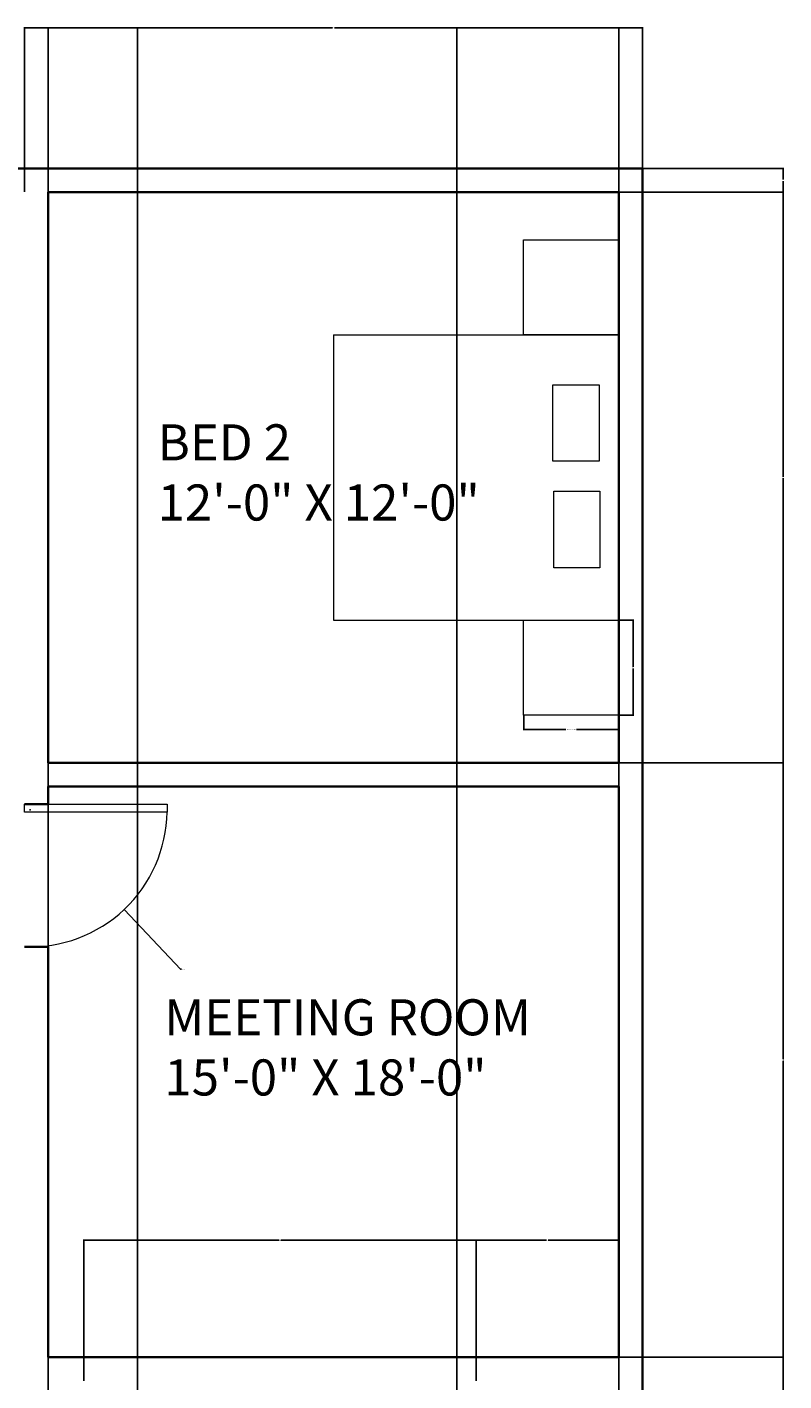
# Model space of a CAD drawing. Units: inches. Extents: x 4468 to 4972, y 2758 to 3538.
# Tile 4 of 4: x 4781 to 4972, y 3196 to 3538. Entities that reach past the tile are written whole.
import ezdxf

# ---------------------------------------------------------------- set-up
doc = ezdxf.new("R2010")
doc.units = ezdxf.units.IN
for name, color, linetype, lineweight in [('A-ANNO-DIMS', 2, 'Continuous', 18), ('A-AREA-IDEN', 7, 'Continuous', 18), ('A-DOOR', 4, 'Continuous', 18), ('A-FURN', 8, 'Continuous', 15), ('A-WALL', 7, 'Continuous', 35)]:
    doc.layers.add(name, color=color, linetype=linetype, lineweight=lineweight)
doc.styles.get("Standard").update_dxf_attribs({"font": 'arial.ttf'})
doc.dimstyles.get("Standard").update_dxf_attribs({"dimtxt": 0.18, "dimasz": 0.18, "dimexe": 0.18, "dimexo": 0.0625, "dimgap": 0.09, "dimtad": 0, "dimtih": 1, "dimtoh": 1, "dimdec": 4, "dimzin": 0, "dimdsep": 46, "dimtxsty": 'Standard', "dimcen": 0.09, "dimadec": 0, "dimazin": 0, "dimtfac": 1, "dimtdec": 4, "dimtofl": 0, "dimtmove": 0, "dimatfit": 3, "dimfxl": 1, "dimtolj": 1, "dimtzin": 0, "dimarcsym": 0})

# ---------------------------------------------------------------- blocks, each defined once
blk = doc.blocks.new('DOOR-LEAF-36IN')
for p, q in [((0, 0), (0, 36)), ((0, 36), (2, 36)), ((2, 36), (2, 0)), ((2, 0), (0, 0))]:
    blk.add_line(p, q)
blk = doc.blocks.new('BED-FRAME-72X72')
for p, q in [((0, 72), (0, 0)), ((0, 72), (72, 72)), ((0, 0), (72, 0))]:
    blk.add_line(p, q)
blk = doc.blocks.new('BED-PILLOW-PAIR')
for points in [[(0, 46.15), (11.65, 46.15), (11.65, 26.85), (0, 26.85)], [(0.18, 19.3), (11.83, 19.3), (11.83, 0), (0.18, 0)]]:
    blk.add_lwpolyline(points, close=True)
blk = doc.blocks.new('NIGHTSTAND-24X24')
blk.add_lwpolyline([(24, 24), (24, 0), (0, 0), (0, 24)], close=True)
blk = doc.blocks.new('*D19')
at = {"layer": 'A-ANNO-DIMS', "color": 0, "lineweight": -2, "transparency": 16777216}
for p, q in [((4906.18, 3364.1), (4906.18, 3360.38)), ((4930.18, 3364.1), (4930.18, 3360.38)), ((4906.36, 3360.56), (4916.8, 3360.56)), ((4930, 3360.56), (4919.55, 3360.56))]:
    blk.add_line(p, q, dxfattribs=at)
at = {"layer": 'A-ANNO-DIMS', "color": 0, "transparency": 16777216}
for points in [[(4906.36, 3360.59), (4906.36, 3360.53), (4906.18, 3360.56)], [(4930, 3360.59), (4930, 3360.53), (4930.18, 3360.56)]]:
    blk.add_solid(points, dxfattribs=at)
at = {"layer": 'Defpoints', "color": 0, "transparency": 16777216}
for p in [(4906.18, 3364.16), (4930.18, 3364.16), (4930.18, 3360.56)]:
    blk.add_point(p, dxfattribs=at)
at = {"layer": 'A-ANNO-DIMS', "color": 0, "transparency": 16777216, "insert": (4918.18, 3360.56), "char_height": 0.18, "attachment_point": 5}
blk.add_mtext('\\A1;NIGHTSTAND 24 TYP.', dxfattribs=at)
blk = doc.blocks.new('*D20')
at = {"layer": 'A-ANNO-DIMS', "color": 0, "lineweight": -2, "transparency": 16777216}
for p, q in [((4930.24, 3388.16), (4933.96, 3388.16)), ((4933.78, 3387.98), (4933.78, 3376.34)), ((4933.78, 3364.34), (4933.78, 3375.98)), ((4930.24, 3364.16), (4933.96, 3364.16))]:
    blk.add_line(p, q, dxfattribs=at)
at = {"layer": 'A-ANNO-DIMS', "color": 0, "transparency": 16777216}
for points in [[(4933.75, 3387.98), (4933.81, 3387.98), (4933.78, 3388.16)], [(4933.75, 3364.34), (4933.81, 3364.34), (4933.78, 3364.16)]]:
    blk.add_solid(points, dxfattribs=at)
at = {"layer": 'Defpoints', "color": 0, "transparency": 16777216}
for p in [(4930.18, 3388.16), (4933.78, 3388.16), (4930.18, 3364.16)]:
    blk.add_point(p, dxfattribs=at)
at = {"layer": 'A-ANNO-DIMS', "color": 0, "transparency": 16777216, "insert": (4933.78, 3376.16), "char_height": 0.18, "attachment_point": 5}
blk.add_mtext('\\A1;24 TYP.', dxfattribs=at)
blk = doc.blocks.new('*D40')
at = {"layer": 'A-ANNO-DIMS', "color": 0, "lineweight": -2, "transparency": 16777216}
for p, q in [((4780.18, 3496.22), (4780.18, 3537.84)), ((4780.36, 3537.66), (4857.9, 3537.66)), ((4936, 3537.66), (4858.46, 3537.66)), ((4936.18, 3502.22), (4936.18, 3537.84))]:
    blk.add_line(p, q, dxfattribs=at)
at = {"layer": 'A-ANNO-DIMS', "color": 0, "transparency": 16777216}
for points in [[(4780.36, 3537.69), (4780.36, 3537.63), (4780.18, 3537.66)], [(4936, 3537.69), (4936, 3537.63), (4936.18, 3537.66)]]:
    blk.add_solid(points, dxfattribs=at)
at = {"layer": 'Defpoints', "color": 0, "transparency": 16777216}
for p in [(4936.18, 3537.66), (4936.18, 3502.16), (4780.18, 3496.16)]:
    blk.add_point(p, dxfattribs=at)
at = {"layer": 'A-ANNO-DIMS', "color": 0, "transparency": 16777216, "insert": (4858.18, 3537.66), "char_height": 0.18, "attachment_point": 5}
blk.add_mtext('\\A1;156', dxfattribs=at)
blk = doc.blocks.new('*D43')
at = {"layer": 'A-ANNO-DIMS', "color": 0, "lineweight": -2, "transparency": 16777216}
for p, q in [((4930.24, 3496.16), (4971.86, 3496.16)), ((4971.68, 3495.98), (4971.68, 3424.34)), ((4971.68, 3352.34), (4971.68, 3423.98)), ((4930.24, 3352.16), (4971.86, 3352.16))]:
    blk.add_line(p, q, dxfattribs=at)
at = {"layer": 'A-ANNO-DIMS', "color": 0, "transparency": 16777216}
for points in [[(4971.65, 3495.98), (4971.71, 3495.98), (4971.68, 3496.16)], [(4971.65, 3352.34), (4971.71, 3352.34), (4971.68, 3352.16)]]:
    blk.add_solid(points, dxfattribs=at)
at = {"layer": 'Defpoints', "color": 0, "transparency": 16777216}
for p in [(4930.18, 3496.16), (4971.68, 3496.16), (4930.18, 3352.16)]:
    blk.add_point(p, dxfattribs=at)
at = {"layer": 'A-ANNO-DIMS', "color": 0, "transparency": 16777216, "insert": (4971.68, 3424.16), "char_height": 0.18, "attachment_point": 5}
blk.add_mtext('\\A1;144', dxfattribs=at)
blk = doc.blocks.new('*D44')
at = {"layer": 'A-ANNO-DIMS', "color": 0, "lineweight": -2, "transparency": 16777216}
for p, q in [((4930.24, 3352.16), (4971.86, 3352.16)), ((4971.68, 3351.98), (4971.68, 3277.34)), ((4971.68, 3202.34), (4971.68, 3276.98)), ((4930.24, 3202.16), (4971.86, 3202.16))]:
    blk.add_line(p, q, dxfattribs=at)
at = {"layer": 'A-ANNO-DIMS', "color": 0, "transparency": 16777216}
for points in [[(4971.65, 3351.98), (4971.71, 3351.98), (4971.68, 3352.16)], [(4971.65, 3202.34), (4971.71, 3202.34), (4971.68, 3202.16)]]:
    blk.add_solid(points, dxfattribs=at)
at = {"layer": 'Defpoints', "color": 0, "transparency": 16777216}
for p in [(4930.18, 3352.16), (4971.68, 3352.16), (4930.18, 3202.16)]:
    blk.add_point(p, dxfattribs=at)
at = {"layer": 'A-ANNO-DIMS', "color": 0, "transparency": 16777216, "insert": (4971.68, 3277.16), "char_height": 0.18, "attachment_point": 5}
blk.add_mtext('\\A1;150', dxfattribs=at)
blk = doc.blocks.new('*D45')
at = {"layer": 'A-ANNO-DIMS', "color": 0, "lineweight": -2, "transparency": 16777216}
for p, q in [((4930.24, 3202.16), (4971.86, 3202.16)), ((4971.68, 3201.98), (4971.68, 3151.34)), ((4971.68, 3100.34), (4971.68, 3150.98)), ((4930.24, 3100.16), (4971.86, 3100.16))]:
    blk.add_line(p, q, dxfattribs=at)
at = {"layer": 'A-ANNO-DIMS', "color": 0, "transparency": 16777216}
for points in [[(4971.65, 3201.98), (4971.71, 3201.98), (4971.68, 3202.16)], [(4971.65, 3100.34), (4971.71, 3100.34), (4971.68, 3100.16)]]:
    blk.add_solid(points, dxfattribs=at)
at = {"layer": 'Defpoints', "color": 0, "transparency": 16777216}
for p in [(4930.18, 3202.16), (4971.68, 3202.16), (4930.18, 3100.16)]:
    blk.add_point(p, dxfattribs=at)
at = {"layer": 'A-ANNO-DIMS', "color": 0, "transparency": 16777216, "insert": (4971.68, 3151.16), "char_height": 0.18, "attachment_point": 5}
blk.add_mtext('\\A1;102', dxfattribs=at)
blk = doc.blocks.new('*D48')
at = {"layer": 'A-ANNO-DIMS', "color": 0, "lineweight": -2, "transparency": 16777216}
for p, q in [((4936.24, 3502.16), (4971.86, 3502.16)), ((4971.68, 3501.98), (4971.68, 3499.34)), ((4971.68, 3496.34), (4971.68, 3498.98)), ((4930.24, 3496.16), (4971.86, 3496.16))]:
    blk.add_line(p, q, dxfattribs=at)
at = {"layer": 'A-ANNO-DIMS', "color": 0, "transparency": 16777216}
for points in [[(4971.65, 3501.98), (4971.71, 3501.98), (4971.68, 3502.16)], [(4971.65, 3496.34), (4971.71, 3496.34), (4971.68, 3496.16)]]:
    blk.add_solid(points, dxfattribs=at)
at = {"layer": 'Defpoints', "color": 0, "transparency": 16777216}
for p in [(4936.18, 3502.16), (4971.68, 3502.16), (4930.18, 3496.16)]:
    blk.add_point(p, dxfattribs=at)
at = {"layer": 'A-ANNO-DIMS', "color": 0, "transparency": 16777216, "insert": (4971.68, 3499.16), "char_height": 0.18, "attachment_point": 5}
blk.add_mtext('\\A1;6', dxfattribs=at)
blk = doc.blocks.new('*D57')
at = {"layer": 'A-ANNO-DIMS', "color": 0, "lineweight": -2, "transparency": 16777216}
for p, q in [((4795.18, 3196.22), (4795.18, 3231.84)), ((4795.36, 3231.66), (4844.46, 3231.66)), ((4894, 3231.66), (4844.89, 3231.66)), ((4894.18, 3196.22), (4894.18, 3231.84))]:
    blk.add_line(p, q, dxfattribs=at)
at = {"layer": 'A-ANNO-DIMS', "color": 0, "transparency": 16777216}
for points in [[(4795.36, 3231.69), (4795.36, 3231.63), (4795.18, 3231.66)], [(4894, 3231.69), (4894, 3231.63), (4894.18, 3231.66)]]:
    blk.add_solid(points, dxfattribs=at)
at = {"layer": 'Defpoints', "color": 0, "transparency": 16777216}
for p in [(4894.18, 3231.66), (4795.18, 3196.16), (4894.18, 3196.16)]:
    blk.add_point(p, dxfattribs=at)
at = {"layer": 'A-ANNO-DIMS', "color": 0, "transparency": 16777216, "insert": (4844.68, 3231.66), "char_height": 0.18, "attachment_point": 5}
blk.add_mtext('\\A1;99', dxfattribs=at)
blk = doc.blocks.new('*D58')
at = {"layer": 'A-ANNO-DIMS', "color": 0, "lineweight": -2, "transparency": 16777216}
for p, q in [((4894.18, 3196.22), (4894.18, 3231.84)), ((4894.36, 3231.66), (4911.96, 3231.66)), ((4930, 3231.66), (4912.39, 3231.66)), ((4930.18, 3196.22), (4930.18, 3231.84))]:
    blk.add_line(p, q, dxfattribs=at)
at = {"layer": 'A-ANNO-DIMS', "color": 0, "transparency": 16777216}
for points in [[(4894.36, 3231.69), (4894.36, 3231.63), (4894.18, 3231.66)], [(4930, 3231.69), (4930, 3231.63), (4930.18, 3231.66)]]:
    blk.add_solid(points, dxfattribs=at)
at = {"layer": 'Defpoints', "color": 0, "transparency": 16777216}
for p in [(4930.18, 3231.66), (4894.18, 3196.16), (4930.18, 3196.16)]:
    blk.add_point(p, dxfattribs=at)
at = {"layer": 'A-ANNO-DIMS', "color": 0, "transparency": 16777216, "insert": (4912.18, 3231.66), "char_height": 0.18, "attachment_point": 5}
blk.add_mtext('\\A1;36', dxfattribs=at)
blk = doc.blocks.new('*D70')
at = {"layer": 'A-ANNO-DIMS', "color": 0, "lineweight": -2, "transparency": 16777216}
for p, q in [((4786.18, 3094.22), (4786.18, 3537.84)), ((4786.36, 3537.66), (4796.95, 3537.66)), ((4808.48, 3537.66), (4797.88, 3537.66)), ((4808.66, 3089.77), (4808.66, 3537.84))]:
    blk.add_line(p, q, dxfattribs=at)
at = {"layer": 'A-ANNO-DIMS', "color": 0, "transparency": 16777216}
for points in [[(4786.36, 3537.69), (4786.36, 3537.63), (4786.18, 3537.66)], [(4808.48, 3537.69), (4808.48, 3537.63), (4808.66, 3537.66)]]:
    blk.add_solid(points, dxfattribs=at)
at = {"layer": 'Defpoints', "color": 0, "transparency": 16777216}
for p in [(4808.66, 3537.66), (4786.18, 3094.16), (4808.66, 3089.71)]:
    blk.add_point(p, dxfattribs=at)
at = {"layer": 'A-ANNO-DIMS', "color": 0, "transparency": 16777216, "insert": (4797.42, 3537.66), "char_height": 0.18, "attachment_point": 5}
blk.add_mtext('\\A1;22.487', dxfattribs=at)
blk = doc.blocks.new('*D71')
at = {"layer": 'A-ANNO-DIMS', "color": 0, "lineweight": -2, "transparency": 16777216}
for p, q in [((4889.29, 3091.63), (4889.29, 3537.84)), ((4889.47, 3537.66), (4909.33, 3537.66)), ((4930, 3537.66), (4910.13, 3537.66)), ((4930.18, 3094.22), (4930.18, 3537.84))]:
    blk.add_line(p, q, dxfattribs=at)
at = {"layer": 'A-ANNO-DIMS', "color": 0, "transparency": 16777216}
for points in [[(4889.47, 3537.69), (4889.47, 3537.63), (4889.29, 3537.66)], [(4930, 3537.69), (4930, 3537.63), (4930.18, 3537.66)]]:
    blk.add_solid(points, dxfattribs=at)
at = {"layer": 'Defpoints', "color": 0, "transparency": 16777216}
for p in [(4930.18, 3537.66), (4930.18, 3094.16), (4889.29, 3091.57)]:
    blk.add_point(p, dxfattribs=at)
at = {"layer": 'A-ANNO-DIMS', "color": 0, "transparency": 16777216, "insert": (4909.73, 3537.66), "char_height": 0.18, "attachment_point": 5}
blk.add_mtext('\\A1;40.89', dxfattribs=at)
blk = doc.blocks.new('*D79')
at = {"layer": 'A-ANNO-DIMS', "color": 0, "lineweight": -2, "transparency": 16777216}
for p, q in [((4781.47, 3340.32), (4781.65, 3340.32)), ((4781.56, 3340.23), (4781.56, 3340.41)), ((4819.59, 3300.04), (4805.45, 3315.01)), ((4819.77, 3300.04), (4819.59, 3300.04))]:
    blk.add_line(p, q, dxfattribs=at)
at = {"layer": 'A-ANNO-DIMS', "color": 0, "transparency": 16777216}
blk.add_solid([(4805.48, 3315.03), (4805.43, 3314.99), (4805.33, 3315.15)], dxfattribs=at)
at = {"layer": 'Defpoints', "color": 0, "transparency": 16777216}
for p in [(4781.56, 3340.32), (4805.33, 3315.15)]:
    blk.add_point(p, dxfattribs=at)
at = {"layer": 'A-ANNO-DIMS', "color": 0, "transparency": 16777216, "insert": (4820.33, 3300.04), "char_height": 0.18, "attachment_point": 5}
blk.add_mtext('\\A1;R34.625', dxfattribs=at)

msp = doc.modelspace()

# ---------------------------------------------------------------- linework, layer by layer
at = {"layer": 'A-DOOR'}
msp.add_arc((4781.5553, 3340.3178), 34.6252, 267.715973, 359.010873, dxfattribs=at)
at = {"layer": 'A-WALL'}
for p, q in [((4504.1753, 3502.1582), (4936.1753, 3502.1582)), ((4936.1753, 3502.1582), (4936.1753, 2794.1582)), ((4786.1753, 3496.1582), (4786.1753, 3352.1582)), ((4786.1753, 3496.1582), (4930.1753, 3496.1582)), ((4930.1753, 3496.1582), (4930.1753, 3352.1582)), ((4786.1753, 3352.1582), (4930.1753, 3352.1582)), ((4786.1753, 3346.1582), (4930.1753, 3346.1582)), ((4786.1753, 3346.1582), (4786.1753, 3341.7201)), ((4930.1753, 3346.1582), (4930.1753, 3202.1582)), ((4780.1753, 3341.7201), (4786.1753, 3341.7201)), ((4780.1753, 3305.7201), (4786.1753, 3305.7201)), ((4786.1753, 3305.7201), (4786.1753, 3202.1582)), ((4786.1753, 3202.1582), (4930.1753, 3202.1582))]:
    msp.add_line(p, q, dxfattribs=at)

# ---------------------------------------------------------------- block references
at = {"layer": 'A-DOOR', "rotation": 270}
msp.add_blockref('DOOR-LEAF-36IN', (4780.1753, 3341.7201), dxfattribs=at)
at = {"layer": 'A-FURN'}
for name, p in [('NIGHTSTAND-24X24', (4906.1753, 3460.1582)), ('BED-FRAME-72X72', (4858.1753, 3388.1582)), ('BED-PILLOW-PAIR', (4913.5783, 3401.3984)), ('NIGHTSTAND-24X24', (4906.1753, 3364.1582))]:
    msp.add_blockref(name, p, dxfattribs=at)

# ---------------------------------------------------------------- texts
at = {"layer": 'A-AREA-IDEN', "char_height": 9.103585, "attachment_point": 1}
for s, insert in [('BED 2\\P12\'-0" X 12\'-0"', (4813.7581, 3437.5784)), ('MEETING ROOM \\P15\'-0" X 18\'-0"', (4815.4825, 3292.4767))]:
    msp.add_mtext_dynamic_manual_height_columns(s, width=327.642018, gutter_width=45.5179, heights=[0], dxfattribs=dict(at, insert=insert))

# ---------------------------------------------------------------- dimensions: what is measured, and where the dimension line sits
at = {"layer": 'A-ANNO-DIMS'}
for base, p1, p2, override, picture, middle in [((4936.1753, 3537.6582), (4780.1753, 3496.1582), (4936.1753, 3502.1582), {"dimdec": 0, "dimlfac": 1, "dimrnd": 0, "dimzin": 0, "dimdsep": 46, "dimlunit": 2}, '*D40', (4858.1753, 3537.6582)), ((4808.6626, 3537.6582), (4786.1753, 3094.1582), (4808.6626, 3089.7108), {"dimdec": 3, "dimlfac": 1, "dimrnd": 0, "dimzin": 0, "dimdsep": 46, "dimlunit": 2}, '*D70', (4797.4189, 3537.6582)), ((4930.1753, 3537.6582), (4889.2887, 3091.5651), (4930.1753, 3094.1582), {"dimdec": 2, "dimlfac": 1, "dimrnd": 0, "dimzin": 0, "dimdsep": 46, "dimlunit": 2}, '*D71', (4909.732, 3537.6582)), ((4894.1753, 3231.6582), (4795.1753, 3196.1582), (4894.1753, 3196.1582), {"dimdec": 0, "dimlfac": 1, "dimrnd": 0, "dimzin": 0, "dimdsep": 46, "dimlunit": 2}, '*D57', (4844.6753, 3231.6582)), ((4930.1753, 3231.6582), (4894.1753, 3196.1582), (4930.1753, 3196.1582), {"dimdec": 0, "dimlfac": 1, "dimrnd": 0, "dimzin": 0, "dimdsep": 46, "dimlunit": 2}, '*D58', (4912.1753, 3231.6582))]:
    dim = msp.add_linear_dim(base=base, p1=p1, p2=p2, dimstyle='Standard', override=override, dxfattribs=at)
    dim.commit()
    dim.dimension.update_dxf_attribs({"geometry": picture, "text_midpoint": middle})
for base, p1, p2, picture, middle in [((4971.6753, 3502.1582), (4930.1753, 3496.1582), (4936.1753, 3502.1582), '*D48', (4971.6753, 3499.1582)), ((4971.6753, 3496.1582), (4930.1753, 3352.1582), (4930.1753, 3496.1582), '*D43', (4971.6753, 3424.1582)), ((4971.6753, 3352.1582), (4930.1753, 3202.1582), (4930.1753, 3352.1582), '*D44', (4971.6753, 3277.1582)), ((4971.6753, 3202.1582), (4930.1753, 3100.1582), (4930.1753, 3202.1582), '*D45', (4971.6753, 3151.1582))]:
    dim = msp.add_linear_dim(base=base, p1=p1, p2=p2, angle=90, dimstyle='Standard', override={"dimdec": 0, "dimlfac": 1, "dimrnd": 0, "dimzin": 0, "dimdsep": 46, "dimlunit": 2}, dxfattribs=at)
    dim.commit()
    dim.dimension.update_dxf_attribs({"geometry": picture, "text_midpoint": middle})
dim = msp.add_linear_dim(base=(4933.7753, 3388.1582), p1=(4930.1753, 3364.1582), p2=(4930.1753, 3388.1582), angle=90, text='<> TYP.', dimstyle='Standard', override={"dimdec": 0, "dimlfac": 1, "dimrnd": 0, "dimzin": 0, "dimdsep": 46, "dimlunit": 2}, dxfattribs=at)
dim.commit()
dim.dimension.update_dxf_attribs({"geometry": '*D20', "text_midpoint": (4933.7753, 3376.1582)})
dim = msp.add_linear_dim(base=(4930.1753, 3360.5582), p1=(4906.1753, 3364.1582), p2=(4930.1753, 3364.1582), text='NIGHTSTAND <> TYP.', dimstyle='Standard', override={"dimdec": 0, "dimlfac": 1, "dimrnd": 0, "dimzin": 0, "dimdsep": 46, "dimlunit": 2}, dxfattribs=at)
dim.commit()
dim.dimension.update_dxf_attribs({"geometry": '*D19', "text_midpoint": (4918.1753, 3360.5582)})
dim = msp.add_radius_dim(center=(4781.5553, 3340.3178), mpoint=(4805.33, 3315.145), dimstyle='Standard', override={"dimdec": 3, "dimlfac": 1, "dimrnd": 0, "dimzin": 0, "dimdsep": 46, "dimlunit": 2}, dxfattribs=at)
dim.commit()
dim.dimension.update_dxf_attribs({"geometry": '*D79', "text_midpoint": (4820.3253, 3300.0413), "dimtype": 164})

doc.saveas('drawing.dxf')
